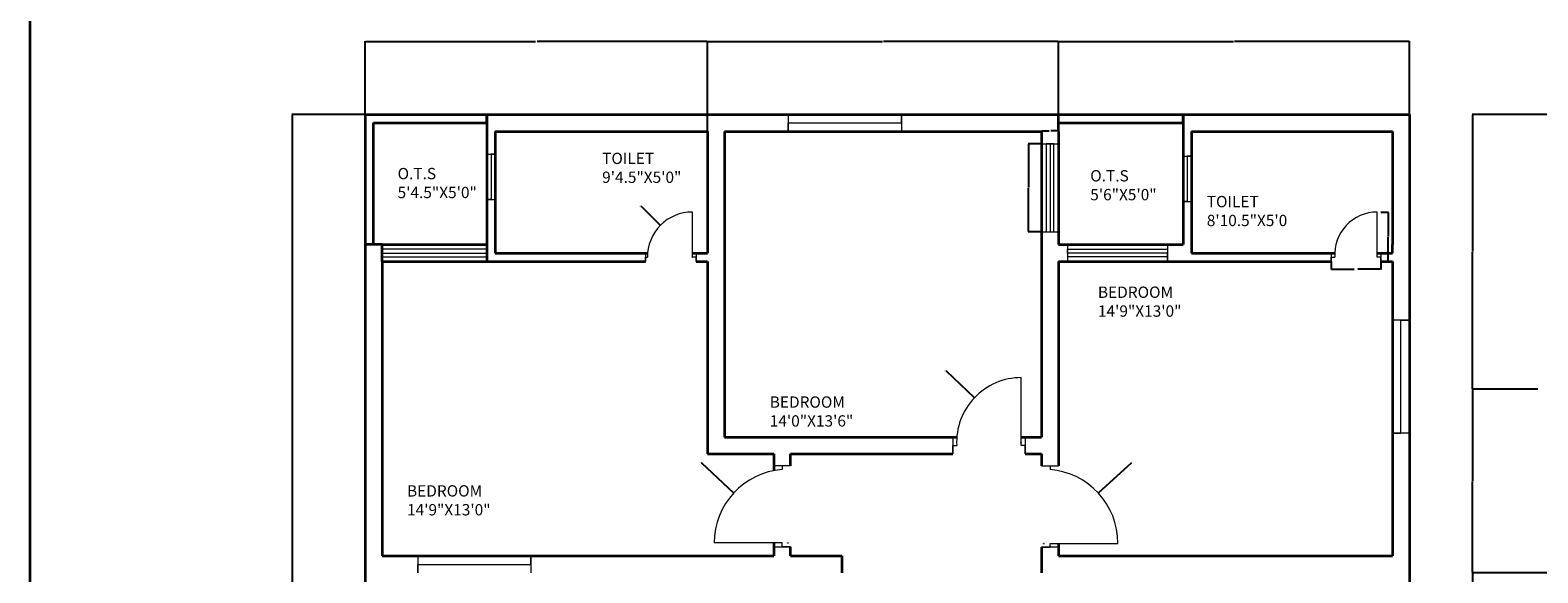
# Model space of a CAD drawing. Units: inches. Extents: x 2014 to 3678, y 870 to 2323.
# Tile 2 of 7: x 2014 to 2813, y 1440 to 1728. Entities that reach past the tile are written whole.
import ezdxf

# ---------------------------------------------------------------- set-up
doc = ezdxf.new("R2010")
doc.units = ezdxf.units.IN
for name, color, linetype, lineweight in [('A-ANNO-DIMS', 2, 'Continuous', 18), ('A-ANNO-TTLB', 7, 'Continuous', 35), ('A-AREA-IDEN', 7, 'Continuous', 18), ('A-DOOR', 3, 'Continuous', 18), ('A-GLAZ', 4, 'Continuous', 18), ('A-WALL', 7, 'Continuous', 35)]:
    doc.layers.add(name, color=color, linetype=linetype, lineweight=lineweight)
doc.styles.get("Standard").update_dxf_attribs({"font": 'arial.ttf'})
doc.dimstyles.get("Standard").update_dxf_attribs({"dimtxt": 0.18, "dimasz": 0.18, "dimexe": 0.18, "dimexo": 0.0625, "dimgap": 0.09, "dimtad": 0, "dimtih": 1, "dimtoh": 1, "dimdec": 4, "dimzin": 0, "dimdsep": 46, "dimtxsty": 'Standard', "dimcen": 0.09, "dimadec": 0, "dimazin": 0, "dimtfac": 1, "dimtdec": 4, "dimtofl": 0, "dimtmove": 0, "dimatfit": 3, "dimfxl": 1, "dimtolj": 1, "dimtzin": 0, "dimarcsym": 0})

# ---------------------------------------------------------------- blocks, each defined once
blk = doc.blocks.new('DOOR-BATH-EAST-24')
for p, q in [((24.34, 2.25), (24.34, 26.25)), ((0, 4.5), (0, 0)), ((0, 0), (0, 2.25)), ((0, 2.25), (2, 2.25)), ((26.34, 2.25), (24.34, 2.25)), ((26.34, 4.5), (26.34, 0)), ((26.34, 0), (26.34, 2.25))]:
    blk.add_line(p, q)
blk.add_arc((24.34, 3.85), 22.4, 90, 184.10271)
blk = doc.blocks.new('DOOR-BATH-WEST-24')
for p, q in [((24.83, 2.25), (24.83, 26.25)), ((0, 4.5), (0, 0)), ((0, 0), (0, 2.25)), ((0, 2.25), (1, 2.25)), ((26.83, 2.25), (24.83, 2.25)), ((26.83, 4.5), (26.83, 0)), ((26.83, 0), (26.83, 2.25))]:
    blk.add_line(p, q)
blk.add_arc((24.83, 2.42), 23.83, 90, 180.40003)
blk = doc.blocks.new('DOOR-BED-CENTRE-36')
for p, q in [((36.22, 28.5), (36.22, 40.5)), ((36.22, 4.5), (36.22, 28.5)), ((0, 9), (0, 0)), ((38.22, 9), (38.22, 0)), ((0, 0), (0, 4.5)), ((0, 4.5), (2, 4.5)), ((38.22, 4.5), (36.22, 4.5)), ((38.22, 0), (38.22, 4.5))]:
    blk.add_line(p, q)
blk.add_arc((36.22, 6.23), 34.27, 90, 182.89802)
blk = doc.blocks.new('DOOR-BED-WEST-36')
for p, q in [((40.5, 42.9), (31.5, 42.9)), ((36, 42.9), (36, 40.9)), ((36, 2), (0, 2)), ((36, 0), (36, 2)), ((31.5, 0), (40.5, 0)), ((40.5, 0), (36, 0))]:
    blk.add_line(p, q)
blk.add_arc((39.02, 2), 39.02, 94.44098, 180)
blk = doc.blocks.new('DOOR-BED-NE-36')
for p, q in [((0, 43.13), (9, 43.13)), ((4.5, 43.13), (4.5, 41.13)), ((9, 0), (0, 0)), ((0, 0), (4.5, 0)), ((4.5, 0), (4.5, 2)), ((4.5, 2), (40.5, 2))]:
    blk.add_line(p, q)
blk.add_arc((1.23, 2), 39.27, 0, 85.2291)
blk = doc.blocks.new('WIN-60')
for p, q in [((0, 9), (0, 0)), ((60, 4.5), (60, 9)), ((60, 9), (60, 0)), ((0, 0), (0, 4.5)), ((0, 4.5), (60, 4.5))]:
    blk.add_line(p, q)
blk = doc.blocks.new('VENT-24')
for p, q in [((0, 24), (4.5, 24)), ((4.5, 24), (2.25, 24)), ((2.25, 24), (2.25, 0)), ((2.25, 0), (0, 0)), ((0, 0), (4.5, 0))]:
    blk.add_line(p, q)
blk = doc.blocks.new('GLAZ-OTS-EAST')
for p, q in [((0, 9), (0, 0)), ((52.91, 9), (52.91, 0)), ((0, 5.5), (0, 6.5)), ((0, 6.5), (52.91, 6.5)), ((0, 4.5), (0, 5.5)), ((52.91, 4.5), (0, 4.5)), ((52.91, 2.5), (0, 2.5)), ((52.91, 6.5), (52.91, 4.5)), ((52.91, 0), (52.91, 4.5)), ((52.91, 4.5), (52.91, 2.5))]:
    blk.add_line(p, q)
blk = doc.blocks.new('GLAZ-OTS-SIDE')
for p, q in [((0, 46.57), (9, 46.57)), ((4.5, 46.57), (2.5, 46.57)), ((2.5, 46.57), (2.5, 0)), ((4.5, 46.57), (4.5, 0)), ((6.5, 46.57), (4.5, 46.57)), ((6.5, 0), (6.5, 46.57)), ((0, 0), (9, 0)), ((4.5, 0), (6.5, 0))]:
    blk.add_line(p, q)
blk = doc.blocks.new('GLAZ-OTS-WEST')
for p, q in [((55.5, 4), (0, 4)), ((0, 4), (0, 2)), ((0, 2), (55.5, 2)), ((0, 2), (0, 0)), ((0, 0), (55.5, 0)), ((55.5, 2), (55.5, 4))]:
    blk.add_line(p, q)
blk = doc.blocks.new('*D34')
at = {"layer": 'A-ANNO-DIMS', "color": 0, "lineweight": -2, "transparency": 16777216}
for p, q in [((2703.55, 1605.1), (2703.55, 1601.03)), ((2703.73, 1601.21), (2715.79, 1601.21)), ((2729.71, 1601.21), (2717.66, 1601.21)), ((2729.89, 1605.1), (2729.89, 1601.03))]:
    blk.add_line(p, q, dxfattribs=at)
at = {"layer": 'A-ANNO-DIMS', "color": 0, "transparency": 16777216}
for points in [[(2703.73, 1601.24), (2703.73, 1601.18), (2703.55, 1601.21)], [(2729.71, 1601.24), (2729.71, 1601.18), (2729.89, 1601.21)]]:
    blk.add_solid(points, dxfattribs=at)
at = {"layer": 'Defpoints', "color": 0, "transparency": 16777216}
for p in [(2703.55, 1605.17), (2729.89, 1605.17), (2729.89, 1601.21)]:
    blk.add_point(p, dxfattribs=at)
at = {"layer": 'A-ANNO-DIMS', "color": 0, "transparency": 16777216, "insert": (2716.72, 1601.21), "char_height": 0.18, "attachment_point": 5}
blk.add_mtext('\\A1;DOOR 26 TYP.', dxfattribs=at)
blk = doc.blocks.new('*D35')
at = {"layer": 'A-ANNO-DIMS', "color": 0, "lineweight": -2, "transparency": 16777216}
for p, q in [((2729.96, 1631.42), (2734.02, 1631.42)), ((2733.84, 1631.24), (2733.84, 1618.47)), ((2733.84, 1605.35), (2733.84, 1618.11)), ((2729.96, 1605.17), (2734.02, 1605.17))]:
    blk.add_line(p, q, dxfattribs=at)
at = {"layer": 'A-ANNO-DIMS', "color": 0, "transparency": 16777216}
for points in [[(2733.81, 1631.24), (2733.87, 1631.24), (2733.84, 1631.42)], [(2733.81, 1605.35), (2733.87, 1605.35), (2733.84, 1605.17)]]:
    blk.add_solid(points, dxfattribs=at)
at = {"layer": 'Defpoints', "color": 0, "transparency": 16777216}
for p in [(2729.89, 1631.42), (2733.84, 1631.42), (2729.89, 1605.17)]:
    blk.add_point(p, dxfattribs=at)
at = {"layer": 'A-ANNO-DIMS', "color": 0, "transparency": 16777216, "insert": (2733.84, 1618.29), "char_height": 0.18, "attachment_point": 5}
blk.add_mtext('\\A1;26 TYP.', dxfattribs=at)
blk = doc.blocks.new('*D58')
at = {"layer": 'A-ANNO-DIMS', "color": 0, "lineweight": -2, "transparency": 16777216}
for p, q in [((2550, 1667.49), (2542.9, 1667.49)), ((2543.08, 1667.31), (2543.08, 1644.39)), ((2543.08, 1621.1), (2543.08, 1644.02)), ((2550, 1620.92), (2542.9, 1620.92))]:
    blk.add_line(p, q, dxfattribs=at)
at = {"layer": 'A-ANNO-DIMS', "color": 0, "transparency": 16777216}
for points in [[(2543.05, 1667.31), (2543.11, 1667.31), (2543.08, 1667.49)], [(2543.05, 1621.1), (2543.11, 1621.1), (2543.08, 1620.92)]]:
    blk.add_solid(points, dxfattribs=at)
at = {"layer": 'Defpoints', "color": 0, "transparency": 16777216}
for p in [(2543.08, 1667.49), (2550.06, 1667.49), (2550.06, 1620.92)]:
    blk.add_point(p, dxfattribs=at)
at = {"layer": 'A-ANNO-DIMS', "color": 0, "transparency": 16777216, "insert": (2543.08, 1644.21), "char_height": 0.18, "attachment_point": 5}
blk.add_mtext('\\A1;GLAZING 47 TYP.', dxfattribs=at)
blk = doc.blocks.new('*D59')
at = {"layer": 'A-ANNO-DIMS', "color": 0, "lineweight": -2, "transparency": 16777216}
for p, q in [((2550.06, 1667.55), (2550.06, 1674.66)), ((2550.24, 1674.48), (2554.1, 1674.48)), ((2558.88, 1674.48), (2555.02, 1674.48)), ((2559.06, 1667.55), (2559.06, 1674.66))]:
    blk.add_line(p, q, dxfattribs=at)
at = {"layer": 'A-ANNO-DIMS', "color": 0, "transparency": 16777216}
for points in [[(2550.24, 1674.51), (2550.24, 1674.45), (2550.06, 1674.48)], [(2558.88, 1674.51), (2558.88, 1674.45), (2559.06, 1674.48)]]:
    blk.add_solid(points, dxfattribs=at)
at = {"layer": 'Defpoints', "color": 0, "transparency": 16777216}
for p in [(2559.06, 1674.48), (2550.06, 1667.49), (2559.06, 1667.49)]:
    blk.add_point(p, dxfattribs=at)
at = {"layer": 'A-ANNO-DIMS', "color": 0, "transparency": 16777216, "insert": (2554.56, 1674.48), "char_height": 0.18, "attachment_point": 5}
blk.add_mtext('\\A1;9 TYP.', dxfattribs=at)
blk = doc.blocks.new('*D87')
at = {"layer": 'A-ANNO-DIMS', "color": 0, "lineweight": -2, "transparency": 16777216}
for p, q in [((2191.5, 1683.17), (2152.68, 1683.17)), ((2152.86, 1682.99), (2152.86, 1341.35)), ((2152.86, 999.35), (2152.86, 1340.98)), ((2191.5, 999.17), (2152.68, 999.17))]:
    blk.add_line(p, q, dxfattribs=at)
at = {"layer": 'A-ANNO-DIMS', "color": 0, "transparency": 16777216}
for points in [[(2152.83, 1682.99), (2152.89, 1682.99), (2152.86, 1683.17)], [(2152.83, 999.35), (2152.89, 999.35), (2152.86, 999.17)]]:
    blk.add_solid(points, dxfattribs=at)
at = {"layer": 'Defpoints', "color": 0, "transparency": 16777216}
for p in [(2152.86, 1683.17), (2191.56, 1683.17), (2191.56, 999.17)]:
    blk.add_point(p, dxfattribs=at)
at = {"layer": 'A-ANNO-DIMS', "color": 0, "transparency": 16777216, "insert": (2152.86, 1341.17), "char_height": 0.18, "attachment_point": 5}
blk.add_mtext('\\A1;684', dxfattribs=at)
blk = doc.blocks.new('*D88')
at = {"layer": 'A-ANNO-DIMS', "color": 0, "lineweight": -2, "transparency": 16777216}
for p, q in [((2191.56, 1683.23), (2191.56, 1722.05)), ((2191.74, 1721.87), (2281.92, 1721.87)), ((2372.88, 1721.87), (2282.7, 1721.87)), ((2373.06, 1674.23), (2373.06, 1722.05))]:
    blk.add_line(p, q, dxfattribs=at)
at = {"layer": 'A-ANNO-DIMS', "color": 0, "transparency": 16777216}
for points in [[(2191.74, 1721.9), (2191.74, 1721.84), (2191.56, 1721.87)], [(2372.88, 1721.9), (2372.88, 1721.84), (2373.06, 1721.87)]]:
    blk.add_solid(points, dxfattribs=at)
at = {"layer": 'Defpoints', "color": 0, "transparency": 16777216}
for p in [(2373.06, 1721.87), (2191.56, 1683.17), (2373.06, 1674.17)]:
    blk.add_point(p, dxfattribs=at)
at = {"layer": 'A-ANNO-DIMS', "color": 0, "transparency": 16777216, "insert": (2282.31, 1721.87), "char_height": 0.18, "attachment_point": 5}
blk.add_mtext('\\A1;181.5', dxfattribs=at)
blk = doc.blocks.new('*D89')
at = {"layer": 'A-ANNO-DIMS', "color": 0, "lineweight": -2, "transparency": 16777216}
for p, q in [((2373.06, 1674.23), (2373.06, 1722.05)), ((2373.24, 1721.87), (2465.78, 1721.87)), ((2558.88, 1721.87), (2466.34, 1721.87)), ((2559.06, 1683.23), (2559.06, 1722.05))]:
    blk.add_line(p, q, dxfattribs=at)
at = {"layer": 'A-ANNO-DIMS', "color": 0, "transparency": 16777216}
for points in [[(2373.24, 1721.9), (2373.24, 1721.84), (2373.06, 1721.87)], [(2558.88, 1721.9), (2558.88, 1721.84), (2559.06, 1721.87)]]:
    blk.add_solid(points, dxfattribs=at)
at = {"layer": 'Defpoints', "color": 0, "transparency": 16777216}
for p in [(2559.06, 1721.87), (2559.06, 1683.17), (2373.06, 1674.17)]:
    blk.add_point(p, dxfattribs=at)
at = {"layer": 'A-ANNO-DIMS', "color": 0, "transparency": 16777216, "insert": (2466.06, 1721.87), "char_height": 0.18, "attachment_point": 5}
blk.add_mtext('\\A1;186', dxfattribs=at)
blk = doc.blocks.new('*D90')
at = {"layer": 'A-ANNO-DIMS', "color": 0, "lineweight": -2, "transparency": 16777216}
for p, q in [((2559.06, 1683.23), (2559.06, 1722.05)), ((2559.24, 1721.87), (2651.78, 1721.87)), ((2744.88, 1721.87), (2652.34, 1721.87)), ((2745.06, 1683.23), (2745.06, 1722.05))]:
    blk.add_line(p, q, dxfattribs=at)
at = {"layer": 'A-ANNO-DIMS', "color": 0, "transparency": 16777216}
for points in [[(2559.24, 1721.9), (2559.24, 1721.84), (2559.06, 1721.87)], [(2744.88, 1721.9), (2744.88, 1721.84), (2745.06, 1721.87)]]:
    blk.add_solid(points, dxfattribs=at)
at = {"layer": 'Defpoints', "color": 0, "transparency": 16777216}
for p in [(2745.06, 1721.87), (2559.06, 1683.17), (2745.06, 1683.17)]:
    blk.add_point(p, dxfattribs=at)
at = {"layer": 'A-ANNO-DIMS', "color": 0, "transparency": 16777216, "insert": (2652.06, 1721.87), "char_height": 0.18, "attachment_point": 5}
blk.add_mtext('\\A1;186', dxfattribs=at)
blk = doc.blocks.new('*D95')
at = {"layer": 'A-ANNO-DIMS', "color": 0, "lineweight": -2, "transparency": 16777216}
for p, q in [((2848.61, 1440.17), (2778.34, 1440.17)), ((2778.52, 1439.99), (2778.52, 1405.85)), ((2778.52, 1371.35), (2778.52, 1405.48)), ((2857.61, 1371.17), (2778.34, 1371.17))]:
    blk.add_line(p, q, dxfattribs=at)
at = {"layer": 'A-ANNO-DIMS', "color": 0, "transparency": 16777216}
for points in [[(2778.49, 1439.99), (2778.55, 1439.99), (2778.52, 1440.17)], [(2778.49, 1371.35), (2778.55, 1371.35), (2778.52, 1371.17)]]:
    blk.add_solid(points, dxfattribs=at)
at = {"layer": 'Defpoints', "color": 0, "transparency": 16777216}
for p in [(2778.52, 1440.17), (2848.67, 1440.17), (2857.67, 1371.17)]:
    blk.add_point(p, dxfattribs=at)
at = {"layer": 'A-ANNO-DIMS', "color": 0, "transparency": 16777216, "insert": (2778.52, 1405.67), "char_height": 0.18, "attachment_point": 5}
blk.add_mtext('\\A1;69', dxfattribs=at)
blk = doc.blocks.new('*D96')
at = {"layer": 'A-ANNO-DIMS', "color": 0, "lineweight": -2, "transparency": 16777216}
for p, q in [((2813.11, 1537.5), (2778.34, 1537.5)), ((2778.52, 1537.32), (2778.52, 1489.01)), ((2778.52, 1440.35), (2778.52, 1488.65)), ((2848.61, 1440.17), (2778.34, 1440.17))]:
    blk.add_line(p, q, dxfattribs=at)
at = {"layer": 'A-ANNO-DIMS', "color": 0, "transparency": 16777216}
for points in [[(2778.49, 1537.32), (2778.55, 1537.32), (2778.52, 1537.5)], [(2778.49, 1440.35), (2778.55, 1440.35), (2778.52, 1440.17)]]:
    blk.add_solid(points, dxfattribs=at)
at = {"layer": 'Defpoints', "color": 0, "transparency": 16777216}
for p in [(2778.52, 1537.5), (2813.17, 1537.5), (2848.67, 1440.17)]:
    blk.add_point(p, dxfattribs=at)
at = {"layer": 'A-ANNO-DIMS', "color": 0, "transparency": 16777216, "insert": (2778.52, 1488.83), "char_height": 0.18, "attachment_point": 5}
blk.add_mtext('\\A1;97.33', dxfattribs=at)
blk = doc.blocks.new('*D97')
at = {"layer": 'A-ANNO-DIMS', "color": 0, "lineweight": -2, "transparency": 16777216}
for p, q in [((2848.61, 1683.17), (2778.34, 1683.17)), ((2778.52, 1682.99), (2778.52, 1610.51)), ((2778.52, 1537.68), (2778.52, 1610.15)), ((2813.11, 1537.5), (2778.34, 1537.5))]:
    blk.add_line(p, q, dxfattribs=at)
at = {"layer": 'A-ANNO-DIMS', "color": 0, "transparency": 16777216}
for points in [[(2778.49, 1682.99), (2778.55, 1682.99), (2778.52, 1683.17)], [(2778.49, 1537.68), (2778.55, 1537.68), (2778.52, 1537.5)]]:
    blk.add_solid(points, dxfattribs=at)
at = {"layer": 'Defpoints', "color": 0, "transparency": 16777216}
for p in [(2778.52, 1683.17), (2848.67, 1683.17), (2813.17, 1537.5)]:
    blk.add_point(p, dxfattribs=at)
at = {"layer": 'A-ANNO-DIMS', "color": 0, "transparency": 16777216, "insert": (2778.52, 1610.33), "char_height": 0.18, "attachment_point": 5}
blk.add_mtext('\\A1;145.67', dxfattribs=at)
blk = doc.blocks.new('*D121')
at = {"layer": 'A-ANNO-DIMS', "color": 0, "lineweight": -2, "transparency": 16777216}
for p, q in [((2597.53, 1498.34), (2580.32, 1482.52)), ((2597.71, 1498.34), (2597.53, 1498.34)), ((2551.2, 1455.81), (2551.38, 1455.81)), ((2551.29, 1455.72), (2551.29, 1455.9))]:
    blk.add_line(p, q, dxfattribs=at)
at = {"layer": 'A-ANNO-DIMS', "color": 0, "transparency": 16777216}
blk.add_solid([(2580.3, 1482.54), (2580.34, 1482.49), (2580.19, 1482.39)], dxfattribs=at)
at = {"layer": 'Defpoints', "color": 0, "transparency": 16777216}
for p in [(2580.19, 1482.39), (2551.29, 1455.81)]:
    blk.add_point(p, dxfattribs=at)
at = {"layer": 'A-ANNO-DIMS', "color": 0, "transparency": 16777216, "insert": (2598.26, 1498.34), "char_height": 0.18, "attachment_point": 5}
blk.add_mtext('\\A1;R39.266', dxfattribs=at)
blk = doc.blocks.new('*D122')
at = {"layer": 'A-ANNO-DIMS', "color": 0, "lineweight": -2, "transparency": 16777216}
for p, q in [((2369.62, 1498.44), (2369.8, 1498.44)), ((2369.8, 1498.44), (2386.85, 1482.66)), ((2415.54, 1456.03), (2415.72, 1456.03)), ((2415.63, 1455.94), (2415.63, 1456.12))]:
    blk.add_line(p, q, dxfattribs=at)
at = {"layer": 'A-ANNO-DIMS', "color": 0, "transparency": 16777216}
blk.add_solid([(2386.87, 1482.68), (2386.83, 1482.64), (2386.98, 1482.54)], dxfattribs=at)
at = {"layer": 'Defpoints', "color": 0, "transparency": 16777216}
for p in [(2386.98, 1482.54), (2415.63, 1456.03)]:
    blk.add_point(p, dxfattribs=at)
at = {"layer": 'A-ANNO-DIMS', "color": 0, "transparency": 16777216, "insert": (2369.14, 1498.44), "char_height": 0.18, "attachment_point": 5}
blk.add_mtext('\\A1;R39.02', dxfattribs=at)
blk = doc.blocks.new('*D124')
at = {"layer": 'A-ANNO-DIMS', "color": 0, "lineweight": -2, "transparency": 16777216}
for p, q in [((2499.42, 1547.17), (2499.6, 1547.17)), ((2499.6, 1547.17), (2514.37, 1533.13)), ((2539.25, 1509.4), (2539.43, 1509.4)), ((2539.34, 1509.31), (2539.34, 1509.49))]:
    blk.add_line(p, q, dxfattribs=at)
at = {"layer": 'A-ANNO-DIMS', "color": 0, "transparency": 16777216}
blk.add_solid([(2514.39, 1533.15), (2514.35, 1533.11), (2514.5, 1533.01)], dxfattribs=at)
at = {"layer": 'Defpoints', "color": 0, "transparency": 16777216}
for p in [(2514.5, 1533.01), (2539.34, 1509.4)]:
    blk.add_point(p, dxfattribs=at)
at = {"layer": 'A-ANNO-DIMS', "color": 0, "transparency": 16777216, "insert": (2498.94, 1547.17), "char_height": 0.18, "attachment_point": 5}
blk.add_mtext('\\A1;R34.27', dxfattribs=at)
blk = doc.blocks.new('*D128')
at = {"layer": 'A-ANNO-DIMS', "color": 0, "lineweight": -2, "transparency": 16777216}
for p, q in [((2337.76, 1634.45), (2337.94, 1634.45)), ((2337.94, 1634.45), (2347.96, 1624.5)), ((2364.91, 1607.58), (2365.09, 1607.58)), ((2365, 1607.49), (2365, 1607.67))]:
    blk.add_line(p, q, dxfattribs=at)
at = {"layer": 'A-ANNO-DIMS', "color": 0, "transparency": 16777216}
blk.add_solid([(2347.98, 1624.52), (2347.94, 1624.48), (2348.09, 1624.38)], dxfattribs=at)
at = {"layer": 'Defpoints', "color": 0, "transparency": 16777216}
for p in [(2348.09, 1624.38), (2365, 1607.58)]:
    blk.add_point(p, dxfattribs=at)
at = {"layer": 'A-ANNO-DIMS', "color": 0, "transparency": 16777216, "insert": (2337.21, 1634.45), "char_height": 0.18, "attachment_point": 5}
blk.add_mtext('\\A1;R23.834', dxfattribs=at)

msp = doc.modelspace()

# ---------------------------------------------------------------- linework, layer by layer
at = {"layer": 'A-ANNO-TTLB'}
msp.add_lwpolyline([(2014.0556, 2323.3638), (3678.0069, 2323.3638), (3678.0069, 869.855), (2014.0556, 869.855)], close=True, dxfattribs=at)
at = {"layer": 'A-WALL'}
for p, q in [((2191.5607, 1683.1655), (2745.0607, 1683.1655)), ((2191.5607, 1683.1655), (2745.0607, 1683.1655)), ((2191.5607, 1683.1655), (2191.5607, 1083.1655)), ((2196.0607, 1614.1655), (2196.0607, 1678.6655)), ((2196.0607, 1678.6655), (2256.0607, 1678.6655)), ((2256.0607, 1678.6655), (2256.0607, 1683.1655)), ((2256.0607, 1683.1655), (2256.0607, 1674.1655)), ((2559.0607, 1678.6655), (2559.0607, 1683.1655)), ((2559.0607, 1674.1655), (2559.0607, 1678.6655)), ((2559.0607, 1678.6655), (2625.0607, 1678.6655)), ((2625.0607, 1678.6655), (2625.0607, 1683.1655)), ((2625.0607, 1683.1655), (2625.0607, 1674.1655)), ((2745.0607, 1683.1655), (2745.0607, 1083.1655)), ((2256.0607, 1674.1655), (2256.0607, 1605.1655)), ((2260.5607, 1674.1655), (2373.0607, 1674.1655)), ((2260.5607, 1674.1655), (2260.5607, 1614.1655)), ((2373.0607, 1674.1655), (2373.0607, 1609.6655)), ((2382.0607, 1674.1655), (2382.0607, 1512.1655)), ((2382.0607, 1674.1655), (2550.0607, 1674.1655)), ((2550.0607, 1674.1655), (2550.0607, 1614.1655)), ((2559.0607, 1674.1655), (2559.0607, 1614.1655)), ((2625.0607, 1674.1655), (2625.0607, 1614.1655)), ((2629.5607, 1674.1655), (2629.5607, 1614.1655)), ((2629.5607, 1674.1655), (2736.0607, 1674.1655)), ((2736.0607, 1674.1655), (2736.0607, 1614.1655)), ((2200.5607, 1614.1655), (2191.5607, 1614.1655)), ((2200.5607, 1614.1655), (2196.0607, 1614.1655)), ((2200.5607, 1614.1655), (2256.0607, 1614.1655)), ((2200.5607, 1605.1655), (2200.5607, 1614.1655)), ((2260.5607, 1614.1655), (2260.5607, 1609.6655)), ((2550.0607, 1620.9201), (2550.0607, 1512.1655)), ((2559.0607, 1614.1655), (2625.0607, 1614.1655)), ((2629.5607, 1614.1655), (2629.5607, 1609.6655)), ((2736.0607, 1609.6655), (2736.0607, 1614.1655)), ((2260.5607, 1609.6655), (2341.2554, 1609.6655)), ((2364.9977, 1609.6655), (2373.0607, 1609.6655)), ((2629.5607, 1609.6655), (2705.5055, 1609.6655)), ((2727.8937, 1609.6655), (2736.0607, 1609.6655)), ((2200.5607, 1605.1655), (2340.1647, 1605.1655)), ((2200.5607, 1605.1655), (2200.5607, 1449.1655)), ((2366.9977, 1605.1655), (2373.0607, 1605.1655)), ((2373.0607, 1605.1655), (2373.0607, 1503.1655)), ((2559.0607, 1605.1655), (2559.0607, 1503.1655)), ((2559.0607, 1605.1655), (2703.5536, 1605.1655)), ((2729.8937, 1605.1655), (2736.0607, 1605.1655)), ((2736.0607, 1605.1655), (2736.0607, 1449.1655)), ((2382.0607, 1512.1655), (2505.1831, 1512.1655)), ((2539.3386, 1512.1655), (2550.0607, 1512.1655)), ((2373.0607, 1503.1655), (2408.1036, 1503.1655)), ((2408.1036, 1503.1655), (2408.1036, 1494.3233)), ((2417.1036, 1496.9379), (2417.1036, 1503.1655)), ((2417.1036, 1503.1655), (2503.115, 1503.1655)), ((2541.3386, 1503.1655), (2550.0607, 1503.1655)), ((2550.0607, 1503.1655), (2550.0607, 1496.9379)), ((2559.0607, 1503.1655), (2559.0607, 1496.9379)), ((2408.1036, 1456.0336), (2408.1036, 1449.1655)), ((2559.0607, 1455.8082), (2559.0607, 1449.1655)), ((2200.5607, 1449.1655), (2408.1036, 1449.1655)), ((2313.0607, 1449.1655), (2322.0607, 1449.1655)), ((2417.1036, 1449.1655), (2417.1036, 1454.0336)), ((2417.1036, 1449.1655), (2444.2554, 1449.1655)), ((2444.2554, 1449.1655), (2444.2554, 1440.1655)), ((2550.0607, 1453.8082), (2550.0607, 1440.1655)), ((2559.0607, 1449.1655), (2736.0607, 1449.1655))]:
    msp.add_line(p, q, dxfattribs=at)

# ---------------------------------------------------------------- block references
at = {"layer": 'A-DOOR'}
for name, p in [('DOOR-BATH-WEST-24', (2340.165, 1605.165)), ('DOOR-BATH-EAST-24', (2703.554, 1605.165)), ('DOOR-BED-CENTRE-36', (2503.115, 1503.165)), ('DOOR-BED-WEST-36', (2376.604, 1454.034)), ('DOOR-BED-NE-36', (2550.061, 1453.808))]:
    msp.add_blockref(name, p, dxfattribs=at)
at = {"layer": 'A-GLAZ'}
for name, p in [('WIN-60', (2415.8151, 1674.165)), ('VENT-24', (2256.061, 1638.0168)), ('GLAZ-OTS-SIDE', (2550.061, 1620.92)), ('VENT-24', (2625.061, 1636.939)), ('GLAZ-OTS-EAST', (2563.91, 1605.165)), ('GLAZ-OTS-WEST', (2200.561, 1607.665)), ('WIN-60', (2219.4692, 1440.165))]:
    msp.add_blockref(name, p, dxfattribs=at)
at = {"layer": 'A-GLAZ', "extrusion": (0, 0, -1), "zscale": -1, "rotation": 90}
msp.add_blockref('WIN-60', (-2736.0602, 1514.14), dxfattribs=at)

# ---------------------------------------------------------------- texts
at = {"layer": 'A-AREA-IDEN', "char_height": 6, "attachment_point": 1}
for s, width, insert in [('TOILET\\P9\'4.5"X5\'0"', 97.694153, (2317.1938, 1662.8522)), ('O.T.S\\P5\'4.5"X5\'0"', 67.386749, (2208.7928, 1654.7854)), ('O.T.S\\P5\'6"X5\'0"', 59.790295, (2575.8748, 1653.6391)), ('TOILET\\P8\'10.5"X5\'0', 59.576444, (2637.6396, 1639.9389)), ('BEDROOM\\P14\'9"X13\'0"', 122.218082, (2579.9522, 1591.9171)), ('BEDROOM\\P14\'0"X13\'6"', 91.604159, (2406.025, 1533.7008)), ('BEDROOM\\P14\'9"X13\'0"', 169.581272, (2213.7851, 1486.6094))]:
    msp.add_mtext_dynamic_manual_height_columns(s, width=width, gutter_width=12.5, heights=[0], dxfattribs=dict(at, insert=insert))

# ---------------------------------------------------------------- dimensions: what is measured, and where the dimension line sits
at = {"layer": 'A-ANNO-DIMS'}
for base, p1, p2, override, picture, middle in [((2373.0607, 1721.8655), (2191.5607, 1683.1655), (2373.0607, 1674.1655), {"dimdec": 1, "dimlfac": 1, "dimrnd": 0, "dimzin": 0, "dimdsep": 46, "dimlunit": 2}, '*D88', (2282.3107, 1721.8655)), ((2559.0607, 1721.8655), (2373.0607, 1674.1655), (2559.0607, 1683.1655), {"dimdec": 0, "dimlfac": 1, "dimrnd": 0, "dimzin": 0, "dimdsep": 46, "dimlunit": 2}, '*D89', (2466.0607, 1721.8655)), ((2745.0607, 1721.8655), (2559.0607, 1683.1655), (2745.0607, 1683.1655), {"dimdec": 0, "dimlfac": 1, "dimrnd": 0, "dimzin": 0, "dimdsep": 46, "dimlunit": 2}, '*D90', (2652.0607, 1721.8655))]:
    dim = msp.add_linear_dim(base=base, p1=p1, p2=p2, dimstyle='Standard', override=override, dxfattribs=at)
    dim.commit()
    dim.dimension.update_dxf_attribs({"geometry": picture, "text_midpoint": middle})
for base, p1, p2, override, picture, middle in [((2152.8607, 1683.1655), (2191.5607, 999.1655), (2191.5607, 1683.1655), {"dimdec": 0, "dimlfac": 1, "dimrnd": 0, "dimzin": 0, "dimdsep": 46, "dimlunit": 2}, '*D87', (2152.8607, 1341.1655)), ((2778.5231, 1683.1655), (2813.1731, 1537.5002), (2848.6718, 1683.1655), {"dimdec": 2, "dimlfac": 1, "dimrnd": 0, "dimzin": 0, "dimdsep": 46, "dimlunit": 2}, '*D97', (2778.5231, 1610.3328)), ((2778.5231, 1537.5002), (2848.6718, 1440.1655), (2813.1731, 1537.5002), {"dimdec": 2, "dimlfac": 1, "dimrnd": 0, "dimzin": 0, "dimdsep": 46, "dimlunit": 2}, '*D96', (2778.5231, 1488.8328)), ((2778.5231, 1440.1655), (2857.6718, 1371.1655), (2848.6718, 1440.1655), {"dimdec": 0, "dimlfac": 1, "dimrnd": 0, "dimzin": 0, "dimdsep": 46, "dimlunit": 2}, '*D95', (2778.5231, 1405.6655))]:
    dim = msp.add_linear_dim(base=base, p1=p1, p2=p2, angle=90, dimstyle='Standard', override=override, dxfattribs=at)
    dim.commit()
    dim.dimension.update_dxf_attribs({"geometry": picture, "text_midpoint": middle})
for base, p1, p2, text, picture, middle in [((2559.0607, 1674.4771), (2550.0607, 1667.4914), (2559.0607, 1667.4914), '<> TYP.', '*D59', (2554.5607, 1674.4771)), ((2729.8937, 1601.2144), (2703.5536, 1605.1655), (2729.8937, 1605.1655), 'DOOR <> TYP.', '*D34', (2716.7237, 1601.2144))]:
    dim = msp.add_linear_dim(base=base, p1=p1, p2=p2, text=text, dimstyle='Standard', override={"dimdec": 0, "dimlfac": 1, "dimrnd": 0, "dimzin": 0, "dimdsep": 46, "dimlunit": 2}, dxfattribs=at)
    dim.commit()
    dim.dimension.update_dxf_attribs({"geometry": picture, "text_midpoint": middle})
for base, p1, p2, text, picture, middle in [((2543.075, 1667.4914), (2550.0607, 1620.9201), (2550.0607, 1667.4914), 'GLAZING <> TYP.', '*D58', (2543.075, 1644.2057)), ((2733.8448, 1631.4155), (2729.8937, 1605.1655), (2729.8937, 1631.4155), '<> TYP.', '*D35', (2733.8448, 1618.2905))]:
    dim = msp.add_linear_dim(base=base, p1=p1, p2=p2, angle=90, text=text, dimstyle='Standard', override={"dimdec": 0, "dimlfac": 1, "dimrnd": 0, "dimzin": 0, "dimdsep": 46, "dimlunit": 2}, dxfattribs=at)
    dim.commit()
    dim.dimension.update_dxf_attribs({"geometry": picture, "text_midpoint": middle})
for center, mpoint, override, picture, middle in [((2364.9977, 1607.5819), (2348.0861, 1624.3759), {"dimdec": 3, "dimlfac": 1, "dimrnd": 0, "dimzin": 0, "dimdsep": 46, "dimlunit": 2}, '*D128', (2337.2098, 1634.4523)), ((2539.3386, 1509.398), (2514.5028, 1533.0082), {"dimdec": 2, "dimlfac": 1, "dimrnd": 0, "dimzin": 0, "dimdsep": 46, "dimlunit": 2}, '*D124', (2498.9415, 1547.1743)), ((2415.6251, 1456.0336), (2386.9841, 1482.5359), {"dimdec": 2, "dimlfac": 1, "dimrnd": 0, "dimzin": 0, "dimdsep": 46, "dimlunit": 2}, '*D122', (2369.1406, 1498.4373)), ((2551.2949, 1455.8082), (2580.1916, 1482.3936), {"dimdec": 3, "dimlfac": 1, "dimrnd": 0, "dimzin": 0, "dimdsep": 46, "dimlunit": 2}, '*D121', (2598.2593, 1498.3449))]:
    dim = msp.add_radius_dim(center=center, mpoint=mpoint, dimstyle='Standard', override=override, dxfattribs=at)
    dim.commit()
    dim.dimension.update_dxf_attribs({"geometry": picture, "text_midpoint": middle, "dimtype": 164})

doc.saveas('drawing.dxf')
